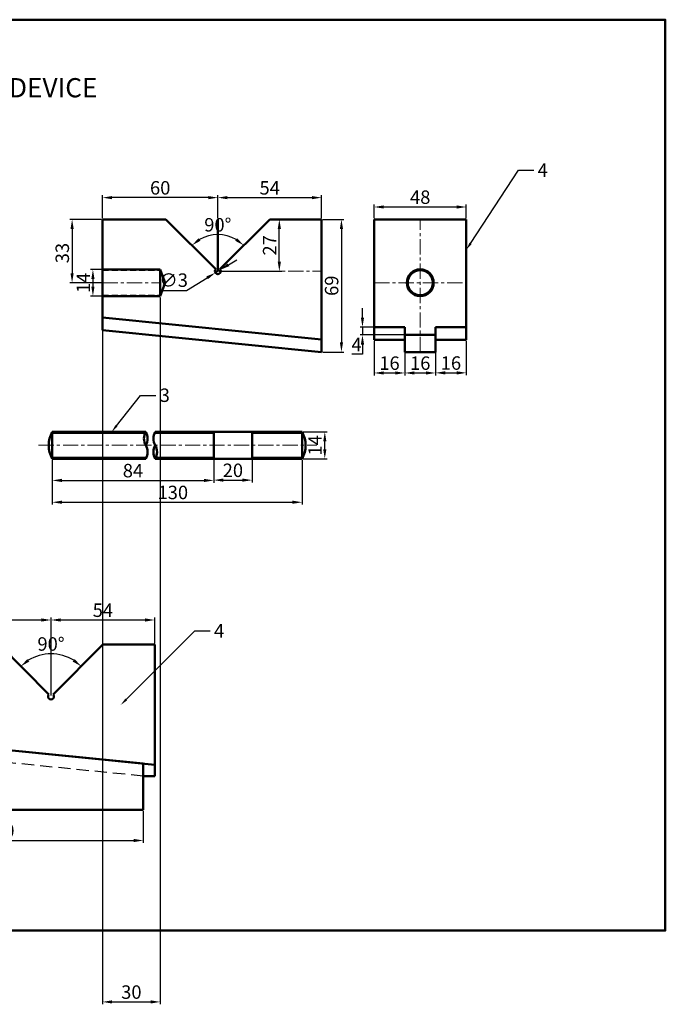
# Model space of a CAD drawing. Units: millimetres. Extents: x -238 to 500, y -191 to 322.
# Tile 3 of 3: x 164 to 500, y -191 to 322. Entities that reach past the tile are written whole.
import ezdxf
from ezdxf import colors
from ezdxf.entities.mleader import LeaderData, LeaderLine
from ezdxf.math import Vec2, Vec3

# ---------------------------------------------------------------- set-up
doc = ezdxf.new("R2010")
doc.units = ezdxf.units.MM
doc.header["$LTSCALE"] = 0.5
doc.linetypes.add('CENTER', pattern=[50.8, 31.75, -6.35, 6.35, -6.35])
doc.linetypes.add('DASHED', pattern=[19.05, 12.7, -6.35])
for name, color, linetype, lineweight in [('M-CNTR', 1, 'CENTER', 18), ('M-DIMS', 2, 'Continuous', 25), ('M-HIDN', 6, 'DASHED', 25), ('M-OUTL', 7, 'Continuous', 50), ('M-TEXT', 3, 'Continuous', 25), ('M-TTLB', 7, 'Continuous', 50)]:
    doc.layers.add(name, color=color, linetype=linetype, lineweight=lineweight)
doc.styles.get("Standard").update_dxf_attribs({"font": 'arial.ttf'})
doc.dimstyles.new('ISO-25', dxfattribs={"dimtxt": 7, "dimasz": 5, "dimexe": 1.25, "dimexo": 0.625, "dimtad": 1, "dimtoh": 1, "dimtxsty": 'Standard', "dimcen": 2.5, "dimadec": 0, "dimazin": 0, "dimtfac": 1, "dimtmove": 0, "dimatfit": 3, "dimfxl": 1, "dimarcsym": 0})

# ---------------------------------------------------------------- blocks, each defined once
blk = doc.blocks.new('*D1')
at = {"layer": 'Defpoints', "color": 0, "ltscale": 0.5, "transparency": 16777216}
for p in [(180.58, 93.15), (310.58, 93.15), (310.58, 70.53)]:
    blk.add_point(p, dxfattribs=at)
at = {"layer": 'M-DIMS', "color": 0, "lineweight": -2, "ltscale": 0.5, "transparency": 16777216}
for p, q in [((180.58, 92.53), (180.58, 69.28)), ((310.58, 92.53), (310.58, 69.28)), ((185.58, 70.53), (305.58, 70.53))]:
    blk.add_line(p, q, dxfattribs=at)
at = {"layer": 'M-DIMS', "color": 0, "ltscale": 0.5, "transparency": 16777216}
for points in [[(185.58, 71.37), (185.58, 69.7), (180.58, 70.53)], [(305.58, 71.37), (305.58, 69.7), (310.58, 70.53)]]:
    blk.add_solid(points, dxfattribs=at)
at = {"layer": 'M-DIMS', "color": 0, "ltscale": 0.5, "transparency": 16777216, "insert": (243.32, 74.73), "char_height": 7, "attachment_point": 5}
blk.add_mtext('130', dxfattribs=at)
blk = doc.blocks.new('*D2')
at = {"layer": 'Defpoints', "color": 0, "ltscale": 0.5, "transparency": 16777216}
for p in [(264.58, 93.15), (284.58, 93.15), (284.58, 82.04)]:
    blk.add_point(p, dxfattribs=at)
at = {"layer": 'M-DIMS', "color": 0, "lineweight": -2, "ltscale": 0.5, "transparency": 16777216}
for p, q in [((264.58, 92.53), (264.58, 80.79)), ((284.58, 92.53), (284.58, 80.79)), ((269.58, 82.04), (279.58, 82.04))]:
    blk.add_line(p, q, dxfattribs=at)
at = {"layer": 'M-DIMS', "color": 0, "ltscale": 0.5, "transparency": 16777216}
for points in [[(269.58, 82.87), (269.58, 81.21), (264.58, 82.04)], [(279.58, 82.87), (279.58, 81.21), (284.58, 82.04)]]:
    blk.add_solid(points, dxfattribs=at)
at = {"layer": 'M-DIMS', "color": 0, "ltscale": 0.5, "transparency": 16777216, "insert": (274.58, 86.24), "char_height": 7, "attachment_point": 5}
blk.add_mtext('20', dxfattribs=at)
blk = doc.blocks.new('*D3')
at = {"layer": 'Defpoints', "color": 0, "ltscale": 0.5, "transparency": 16777216}
for p in [(180.58, 93.15), (264.58, 93.15), (264.58, 81.89)]:
    blk.add_point(p, dxfattribs=at)
at = {"layer": 'M-DIMS', "color": 0, "lineweight": -2, "ltscale": 0.5, "transparency": 16777216}
for p, q in [((180.58, 92.53), (180.58, 80.64)), ((264.58, 92.53), (264.58, 80.64)), ((185.58, 81.89), (259.58, 81.89))]:
    blk.add_line(p, q, dxfattribs=at)
at = {"layer": 'M-DIMS', "color": 0, "ltscale": 0.5, "transparency": 16777216}
for points in [[(185.58, 82.72), (185.58, 81.05), (180.58, 81.89)], [(259.58, 82.72), (259.58, 81.05), (264.58, 81.89)]]:
    blk.add_solid(points, dxfattribs=at)
at = {"layer": 'M-DIMS', "color": 0, "ltscale": 0.5, "transparency": 16777216, "insert": (222.58, 86.08), "char_height": 7, "attachment_point": 5}
blk.add_mtext('84', dxfattribs=at)
blk = doc.blocks.new('*D4')
at = {"layer": 'Defpoints', "color": 0, "ltscale": 0.5, "transparency": 16777216}
for p in [(310.58, 107.15), (322.41, 107.15), (310.58, 93.15)]:
    blk.add_point(p, dxfattribs=at)
at = {"layer": 'M-DIMS', "color": 0, "lineweight": -2, "ltscale": 0.5, "transparency": 16777216}
for p, q in [((311.21, 107.15), (323.66, 107.15)), ((322.41, 98.15), (322.41, 102.15)), ((311.21, 93.15), (323.66, 93.15))]:
    blk.add_line(p, q, dxfattribs=at)
at = {"layer": 'M-DIMS', "color": 0, "ltscale": 0.5, "transparency": 16777216}
for points in [[(321.58, 102.15), (323.25, 102.15), (322.41, 107.15)], [(321.58, 98.15), (323.25, 98.15), (322.41, 93.15)]]:
    blk.add_solid(points, dxfattribs=at)
at = {"layer": 'M-DIMS', "color": 0, "ltscale": 0.5, "transparency": 16777216, "insert": (318.27, 100.15), "char_height": 7, "attachment_point": 5, "rotation": 90}
blk.add_mtext('14', dxfattribs=at)
blk = doc.blocks.new('*D32')
at = {"layer": 'Defpoints', "color": 0, "ltscale": 0.5, "transparency": 16777216}
for p in [(239.74, 217.71), (293.74, 217.71), (271.69, 209.15), (266.74, 190.71), (266.74, 190.71)]:
    blk.add_point(p, dxfattribs=at)
at = {"layer": 'M-DIMS', "color": 0, "lineweight": -2, "ltscale": 0.5, "transparency": 16777216}
blk.add_arc((266.74, 190.71), 19.09, 60.0485, 119.9515, dxfattribs=at)
at = {"layer": 'M-DIMS', "color": 0, "ltscale": 0.5, "transparency": 16777216}
for points in [[(257.72, 206.59), (256.71, 207.92), (253.24, 204.21)], [(276.78, 207.92), (275.77, 206.59), (280.24, 204.21)]]:
    blk.add_solid(points, dxfattribs=at)
at = {"layer": 'M-DIMS', "color": 0, "ltscale": 0.5, "transparency": 16777216, "insert": (266.74, 214), "char_height": 7, "attachment_point": 5}
blk.add_mtext('90°', dxfattribs=at)
blk = doc.blocks.new('*D33')
at = {"layer": 'Defpoints', "color": 0, "ltscale": 0.5, "transparency": 16777216}
for p in [(206.74, 229.03), (206.74, 217.71), (266.74, 217.71)]:
    blk.add_point(p, dxfattribs=at)
at = {"layer": 'M-DIMS', "color": 0, "lineweight": -2, "ltscale": 0.5, "transparency": 16777216}
for p, q in [((206.74, 218.34), (206.74, 230.28)), ((261.74, 229.03), (211.74, 229.03)), ((266.74, 218.34), (266.74, 230.28))]:
    blk.add_line(p, q, dxfattribs=at)
at = {"layer": 'M-DIMS', "color": 0, "ltscale": 0.5, "transparency": 16777216}
for points in [[(211.74, 229.87), (211.74, 228.2), (206.74, 229.03)], [(261.74, 229.87), (261.74, 228.2), (266.74, 229.03)]]:
    blk.add_solid(points, dxfattribs=at)
at = {"layer": 'M-DIMS', "color": 0, "ltscale": 0.5, "transparency": 16777216, "insert": (236.74, 233.23), "char_height": 7, "attachment_point": 5}
blk.add_mtext('60', dxfattribs=at)
blk = doc.blocks.new('*D34')
at = {"layer": 'Defpoints', "color": 0, "ltscale": 0.5, "transparency": 16777216}
for p in [(320.74, 229.03), (266.74, 217.71), (320.74, 217.71)]:
    blk.add_point(p, dxfattribs=at)
at = {"layer": 'M-DIMS', "color": 0, "lineweight": -2, "ltscale": 0.5, "transparency": 16777216}
for p, q in [((266.74, 218.34), (266.74, 230.28)), ((271.74, 229.03), (315.74, 229.03)), ((320.74, 218.34), (320.74, 230.28))]:
    blk.add_line(p, q, dxfattribs=at)
at = {"layer": 'M-DIMS', "color": 0, "ltscale": 0.5, "transparency": 16777216}
for points in [[(271.74, 229.87), (271.74, 228.2), (266.74, 229.03)], [(315.74, 229.87), (315.74, 228.2), (320.74, 229.03)]]:
    blk.add_solid(points, dxfattribs=at)
at = {"layer": 'M-DIMS', "color": 0, "ltscale": 0.5, "transparency": 16777216, "insert": (293.74, 233.22), "char_height": 7, "attachment_point": 5}
blk.add_mtext('54', dxfattribs=at)
blk = doc.blocks.new('*D35')
at = {"layer": 'Defpoints', "color": 0, "ltscale": 0.5, "transparency": 16777216}
for p in [(206.74, 217.71), (190.9, 184.71), (206.74, 184.71)]:
    blk.add_point(p, dxfattribs=at)
at = {"layer": 'M-DIMS', "color": 0, "lineweight": -2, "ltscale": 0.5, "transparency": 16777216}
for p, q in [((206.12, 217.71), (189.65, 217.71)), ((190.9, 212.71), (190.9, 189.71)), ((206.12, 184.71), (189.65, 184.71))]:
    blk.add_line(p, q, dxfattribs=at)
at = {"layer": 'M-DIMS', "color": 0, "ltscale": 0.5, "transparency": 16777216}
for points in [[(190.06, 212.71), (191.73, 212.71), (190.9, 217.71)], [(190.06, 189.71), (191.73, 189.71), (190.9, 184.71)]]:
    blk.add_solid(points, dxfattribs=at)
at = {"layer": 'M-DIMS', "color": 0, "ltscale": 0.5, "transparency": 16777216, "insert": (186.7, 200.19), "char_height": 7, "attachment_point": 5, "rotation": 90}
blk.add_mtext('33', dxfattribs=at)
blk = doc.blocks.new('*D36')
at = {"layer": 'Defpoints', "color": 0, "ltscale": 0.5, "transparency": 16777216}
for p in [(206.74, 191.71), (201.73, 177.71), (206.74, 177.71)]:
    blk.add_point(p, dxfattribs=at)
at = {"layer": 'M-DIMS', "color": 0, "lineweight": -2, "ltscale": 0.5, "transparency": 16777216}
for p, q in [((206.12, 191.71), (200.48, 191.71)), ((201.73, 186.71), (201.73, 182.71)), ((206.12, 177.71), (200.48, 177.71))]:
    blk.add_line(p, q, dxfattribs=at)
at = {"layer": 'M-DIMS', "color": 0, "ltscale": 0.5, "transparency": 16777216}
for points in [[(200.9, 186.71), (202.57, 186.71), (201.73, 191.71)], [(200.9, 182.71), (202.57, 182.71), (201.73, 177.71)]]:
    blk.add_solid(points, dxfattribs=at)
at = {"layer": 'M-DIMS', "color": 0, "ltscale": 0.5, "transparency": 16777216, "insert": (197.6, 184.71), "char_height": 7, "attachment_point": 5, "rotation": 90}
blk.add_mtext('14', dxfattribs=at)
blk = doc.blocks.new('*D37')
at = {"layer": 'Defpoints', "color": 0, "ltscale": 0.5, "transparency": 16777216}
for p in [(320.74, 217.71), (320.74, 148.71), (331.08, 148.71)]:
    blk.add_point(p, dxfattribs=at)
at = {"layer": 'M-DIMS', "color": 0, "lineweight": -2, "ltscale": 0.5, "transparency": 16777216}
for p, q in [((321.37, 217.71), (332.33, 217.71)), ((331.08, 212.71), (331.08, 153.71)), ((321.37, 148.71), (332.33, 148.71))]:
    blk.add_line(p, q, dxfattribs=at)
at = {"layer": 'M-DIMS', "color": 0, "ltscale": 0.5, "transparency": 16777216}
for points in [[(330.24, 212.71), (331.91, 212.71), (331.08, 217.71)], [(330.24, 153.71), (331.91, 153.71), (331.08, 148.71)]]:
    blk.add_solid(points, dxfattribs=at)
at = {"layer": 'M-DIMS', "color": 0, "ltscale": 0.5, "transparency": 16777216, "insert": (326.88, 183.21), "char_height": 7, "attachment_point": 5, "rotation": 90}
blk.add_mtext('69', dxfattribs=at)
blk = doc.blocks.new('*D38')
at = {"layer": 'Defpoints', "color": 0, "ltscale": 0.5, "transparency": 16777216}
for p in [(293.74, 217.71), (298.75, 217.71), (266.74, 190.71)]:
    blk.add_point(p, dxfattribs=at)
at = {"layer": 'M-DIMS', "color": 0, "lineweight": -2, "ltscale": 0.5, "transparency": 16777216}
for p, q in [((294.37, 217.71), (300, 217.71)), ((298.75, 195.71), (298.75, 212.71)), ((267.37, 190.71), (300, 190.71))]:
    blk.add_line(p, q, dxfattribs=at)
at = {"layer": 'M-DIMS', "color": 0, "ltscale": 0.5, "transparency": 16777216}
for points in [[(297.92, 212.71), (299.59, 212.71), (298.75, 217.71)], [(297.92, 195.71), (299.59, 195.71), (298.75, 190.71)]]:
    blk.add_solid(points, dxfattribs=at)
at = {"layer": 'M-DIMS', "color": 0, "ltscale": 0.5, "transparency": 16777216, "insert": (294.61, 204.21), "char_height": 7, "attachment_point": 5, "rotation": 90}
blk.add_mtext('27', dxfattribs=at)
blk = doc.blocks.new('*D39')
at = {"layer": 'Defpoints', "color": 0, "ltscale": 0.5, "transparency": 16777216}
for p in [(265.46, 189.93), (268.03, 191.49)]:
    blk.add_point(p, dxfattribs=at)
at = {"layer": 'M-DIMS', "color": 0, "lineweight": -2, "ltscale": 0.5, "transparency": 16777216}
for p, q in [((272.29, 194.1), (276.56, 196.7)), ((268.03, 191.49), (265.46, 189.93)), ((250.49, 180.8), (261.2, 187.33)), ((237.66, 180.8), (250.49, 180.8))]:
    blk.add_line(p, q, dxfattribs=at)
at = {"layer": 'M-DIMS', "color": 0, "ltscale": 0.5, "transparency": 16777216}
for points in [[(271.86, 194.81), (272.73, 193.39), (268.03, 191.49)], [(260.76, 188.04), (261.63, 186.62), (265.46, 189.93)]]:
    blk.add_solid(points, dxfattribs=at)
at = {"layer": 'M-DIMS', "color": 0, "ltscale": 0.5, "transparency": 16777216, "insert": (243.76, 185.2), "char_height": 7, "attachment_point": 5}
blk.add_mtext('∅3', dxfattribs=at)
blk = doc.blocks.new('*D40')
at = {"layer": 'Defpoints', "color": 0, "ltscale": 0.5, "transparency": 16777216}
for p in [(396.08, 224.17), (348.08, 217.71), (396.08, 217.71)]:
    blk.add_point(p, dxfattribs=at)
at = {"layer": 'M-DIMS', "color": 0, "lineweight": -2, "ltscale": 0.5, "transparency": 16777216}
for p, q in [((348.08, 218.34), (348.08, 225.42)), ((353.08, 224.17), (391.08, 224.17)), ((396.08, 218.34), (396.08, 225.42))]:
    blk.add_line(p, q, dxfattribs=at)
at = {"layer": 'M-DIMS', "color": 0, "ltscale": 0.5, "transparency": 16777216}
for points in [[(353.08, 225.01), (353.08, 223.34), (348.08, 224.17)], [(391.08, 225.01), (391.08, 223.34), (396.08, 224.17)]]:
    blk.add_solid(points, dxfattribs=at)
at = {"layer": 'M-DIMS', "color": 0, "ltscale": 0.5, "transparency": 16777216, "insert": (372.08, 228.37), "char_height": 7, "attachment_point": 5}
blk.add_mtext('48', dxfattribs=at)
blk = doc.blocks.new('*D41')
at = {"layer": 'Defpoints', "color": 0, "ltscale": 0.5, "transparency": 16777216}
for p in [(348.08, 161.58), (342.02, 157.58), (364.08, 157.58)]:
    blk.add_point(p, dxfattribs=at)
at = {"layer": 'M-DIMS', "color": 0, "lineweight": -2, "ltscale": 0.5, "transparency": 16777216}
for p, q in [((342.02, 166.58), (342.02, 171.58)), ((347.45, 161.58), (340.77, 161.58)), ((342.02, 161.58), (342.02, 157.58)), ((363.45, 157.58), (340.77, 157.58)), ((342.02, 152.58), (342.02, 147.58)), ((342.02, 147.58), (336.56, 147.58))]:
    blk.add_line(p, q, dxfattribs=at)
at = {"layer": 'M-DIMS', "color": 0, "ltscale": 0.5, "transparency": 16777216}
for points in [[(341.19, 166.58), (342.86, 166.58), (342.02, 161.58)], [(341.19, 152.58), (342.86, 152.58), (342.02, 157.58)]]:
    blk.add_solid(points, dxfattribs=at)
at = {"layer": 'M-DIMS', "color": 0, "ltscale": 0.5, "transparency": 16777216, "insert": (338.98, 151.71), "char_height": 7, "attachment_point": 5}
blk.add_mtext('4', dxfattribs=at)
blk = doc.blocks.new('*D42')
at = {"layer": 'Defpoints', "color": 0, "ltscale": 0.5, "transparency": 16777216}
for p in [(348.08, 155.08), (364.08, 155.08), (364.08, 137.8)]:
    blk.add_point(p, dxfattribs=at)
at = {"layer": 'M-DIMS', "color": 0, "lineweight": -2, "ltscale": 0.5, "transparency": 16777216}
for p, q in [((348.08, 154.46), (348.08, 136.55)), ((364.08, 154.46), (364.08, 136.55)), ((353.08, 137.8), (359.08, 137.8))]:
    blk.add_line(p, q, dxfattribs=at)
at = {"layer": 'M-DIMS', "color": 0, "ltscale": 0.5, "transparency": 16777216}
for points in [[(353.08, 138.64), (353.08, 136.97), (348.08, 137.8)], [(359.08, 138.64), (359.08, 136.97), (364.08, 137.8)]]:
    blk.add_solid(points, dxfattribs=at)
at = {"layer": 'M-DIMS', "color": 0, "ltscale": 0.5, "transparency": 16777216, "insert": (356.08, 142), "char_height": 7, "attachment_point": 5}
blk.add_mtext('16', dxfattribs=at)
blk = doc.blocks.new('*D43')
at = {"layer": 'Defpoints', "color": 0, "ltscale": 0.5, "transparency": 16777216}
for p in [(364.08, 148.71), (380.08, 148.71), (380.08, 137.8)]:
    blk.add_point(p, dxfattribs=at)
at = {"layer": 'M-DIMS', "color": 0, "lineweight": -2, "ltscale": 0.5, "transparency": 16777216}
for p, q in [((364.08, 148.09), (364.08, 136.55)), ((380.08, 148.09), (380.08, 136.55)), ((369.08, 137.8), (375.08, 137.8))]:
    blk.add_line(p, q, dxfattribs=at)
at = {"layer": 'M-DIMS', "color": 0, "ltscale": 0.5, "transparency": 16777216}
for points in [[(369.08, 138.64), (369.08, 136.97), (364.08, 137.8)], [(375.08, 138.64), (375.08, 136.97), (380.08, 137.8)]]:
    blk.add_solid(points, dxfattribs=at)
at = {"layer": 'M-DIMS', "color": 0, "ltscale": 0.5, "transparency": 16777216, "insert": (372.08, 142), "char_height": 7, "attachment_point": 5}
blk.add_mtext('16', dxfattribs=at)
blk = doc.blocks.new('*D44')
at = {"layer": 'Defpoints', "color": 0, "ltscale": 0.5, "transparency": 16777216}
for p in [(380.08, 155.15), (396.08, 155.15), (396.08, 137.86)]:
    blk.add_point(p, dxfattribs=at)
at = {"layer": 'M-DIMS', "color": 0, "lineweight": -2, "ltscale": 0.5, "transparency": 16777216}
for p, q in [((380.08, 154.52), (380.08, 136.61)), ((396.08, 154.52), (396.08, 136.61)), ((385.08, 137.86), (391.08, 137.86))]:
    blk.add_line(p, q, dxfattribs=at)
at = {"layer": 'M-DIMS', "color": 0, "ltscale": 0.5, "transparency": 16777216}
for points in [[(385.08, 138.69), (385.08, 137.02), (380.08, 137.86)], [(391.08, 138.69), (391.08, 137.02), (396.08, 137.86)]]:
    blk.add_solid(points, dxfattribs=at)
at = {"layer": 'M-DIMS', "color": 0, "ltscale": 0.5, "transparency": 16777216, "insert": (388.08, 142.06), "char_height": 7, "attachment_point": 5}
blk.add_mtext('16', dxfattribs=at)
blk = doc.blocks.new('*D48')
at = {"layer": 'Defpoints', "color": 0, "ltscale": 0.5, "transparency": 16777216}
for p in [(77.97, -89.46), (227.97, -89.46), (227.97, -105.49)]:
    blk.add_point(p, dxfattribs=at)
at = {"layer": 'M-DIMS', "color": 0, "lineweight": -2, "ltscale": 0.5, "transparency": 16777216}
for p, q in [((77.97, -90.09), (77.97, -106.74)), ((227.97, -90.09), (227.97, -106.74)), ((82.97, -105.49), (222.97, -105.49))]:
    blk.add_line(p, q, dxfattribs=at)
at = {"layer": 'M-DIMS', "color": 0, "ltscale": 0.5, "transparency": 16777216}
for points in [[(82.97, -104.66), (82.97, -106.32), (77.97, -105.49)], [(222.97, -104.66), (222.97, -106.32), (227.97, -105.49)]]:
    blk.add_solid(points, dxfattribs=at)
at = {"layer": 'M-DIMS', "color": 0, "ltscale": 0.5, "transparency": 16777216, "insert": (152.97, -101.29), "char_height": 7, "attachment_point": 5}
blk.add_mtext('150', dxfattribs=at)
blk = doc.blocks.new('*D49')
at = {"layer": 'Defpoints', "color": 0, "ltscale": 0.5, "transparency": 16777216}
for p in [(152.92, -3.57), (206.92, -3.57), (185.67, -9.09), (178.86, -29.51), (180.98, -29.51)]:
    blk.add_point(p, dxfattribs=at)
at = {"layer": 'M-DIMS', "color": 0, "lineweight": -2, "ltscale": 0.5, "transparency": 16777216}
blk.add_arc((179.92, -30.57), 22.24, 57.9107, 122.0893, dxfattribs=at)
at = {"layer": 'M-DIMS', "color": 0, "ltscale": 0.5, "transparency": 16777216}
for points in [[(168.62, -12.38), (167.58, -11.08), (164.19, -14.85)], [(192.25, -11.08), (191.21, -12.38), (195.64, -14.85)]]:
    blk.add_solid(points, dxfattribs=at)
at = {"layer": 'M-DIMS', "color": 0, "ltscale": 0.5, "transparency": 16777216, "insert": (179.92, -4.14), "char_height": 7, "attachment_point": 5}
blk.add_mtext('90°', dxfattribs=at)
blk = doc.blocks.new('*D50')
at = {"layer": 'Defpoints', "color": 0, "ltscale": 0.5, "transparency": 16777216}
for p in [(179.92, 9.26), (119.92, -3.57), (179.92, -30.57)]:
    blk.add_point(p, dxfattribs=at)
at = {"layer": 'M-DIMS', "color": 0, "lineweight": -2, "ltscale": 0.5, "transparency": 16777216}
for p, q in [((119.92, -2.95), (119.92, 10.51)), ((179.92, -29.95), (179.92, 10.51)), ((124.92, 9.26), (174.92, 9.26))]:
    blk.add_line(p, q, dxfattribs=at)
at = {"layer": 'M-DIMS', "color": 0, "ltscale": 0.5, "transparency": 16777216}
for points in [[(124.92, 10.09), (124.92, 8.42), (119.92, 9.26)], [(174.92, 10.09), (174.92, 8.42), (179.92, 9.26)]]:
    blk.add_solid(points, dxfattribs=at)
at = {"layer": 'M-DIMS', "color": 0, "ltscale": 0.5, "transparency": 16777216, "insert": (149.92, 13.46), "char_height": 7, "attachment_point": 5}
blk.add_mtext('60', dxfattribs=at)
blk = doc.blocks.new('*D51')
at = {"layer": 'Defpoints', "color": 0, "ltscale": 0.5, "transparency": 16777216}
for p in [(179.92, 9.26), (233.92, 9.26), (233.92, -3.57)]:
    blk.add_point(p, dxfattribs=at)
at = {"layer": 'M-DIMS', "color": 0, "lineweight": -2, "ltscale": 0.5, "transparency": 16777216}
for p, q in [((179.92, 9.88), (179.92, 10.51)), ((233.92, -2.95), (233.92, 10.51)), ((184.92, 9.26), (228.92, 9.26))]:
    blk.add_line(p, q, dxfattribs=at)
at = {"layer": 'M-DIMS', "color": 0, "ltscale": 0.5, "transparency": 16777216}
for points in [[(184.92, 10.09), (184.92, 8.42), (179.92, 9.26)], [(228.92, 10.09), (228.92, 8.42), (233.92, 9.26)]]:
    blk.add_solid(points, dxfattribs=at)
at = {"layer": 'M-DIMS', "color": 0, "ltscale": 0.5, "transparency": 16777216, "insert": (206.92, 13.44), "char_height": 7, "attachment_point": 5}
blk.add_mtext('54', dxfattribs=at)
blk = doc.blocks.new('*D53')
at = {"layer": 'Defpoints', "color": 0, "ltscale": 0.5, "transparency": 16777216}
for p in [(206.74, 177.71), (236.74, 177.71), (236.74, -189.48)]:
    blk.add_point(p, dxfattribs=at)
at = {"layer": 'M-DIMS', "color": 0, "lineweight": -2, "ltscale": 0.5, "transparency": 16777216}
for p, q in [((206.74, 177.09), (206.74, -190.73)), ((236.74, 177.09), (236.74, -190.73)), ((211.74, -189.48), (231.74, -189.48))]:
    blk.add_line(p, q, dxfattribs=at)
at = {"layer": 'M-DIMS', "color": 0, "ltscale": 0.5, "transparency": 16777216}
for points in [[(211.74, -188.65), (211.74, -190.31), (206.74, -189.48)], [(231.74, -188.65), (231.74, -190.31), (236.74, -189.48)]]:
    blk.add_solid(points, dxfattribs=at)
at = {"layer": 'M-DIMS', "color": 0, "ltscale": 0.5, "transparency": 16777216, "insert": (221.74, -185.28), "char_height": 7, "attachment_point": 5}
blk.add_mtext('30', dxfattribs=at)

msp = doc.modelspace()

# ---------------------------------------------------------------- linework, layer by layer
at = {"layer": 'M-CNTR', "ltscale": 0.5}
for p, q in [((372.077, 148.713), (372.077, 217.713)), ((265.245, 190.713), (320.745, 190.713)), ((206.745, 184.713), (236.745, 184.713)), ((348.077, 184.713), (396.077, 184.713)), ((173.464, 100.152), (318.355, 100.152))]:
    msp.add_line(p, q, dxfattribs=at)
at = {"layer": 'M-HIDN', "ltscale": 0.5}
for p, q in [((206.745, 191.213), (236.745, 191.213)), ((206.745, 178.213), (236.745, 178.213))]:
    msp.add_line(p, q, dxfattribs=at)
at = {"layer": 'M-HIDN'}
msp.add_line((227.969, -71.997), (119.916, -61.193), dxfattribs=at)
at = {"layer": 'M-OUTL', "ltscale": 0.5}
for p, q in [((206.745, 217.713), (239.745, 217.713)), ((206.745, 217.713), (206.745, 184.713)), ((265.684, 191.774), (239.745, 217.713)), ((266.745, 217.713), (266.745, 190.713)), ((267.805, 191.774), (293.745, 217.713)), ((293.745, 217.713), (320.745, 217.713)), ((320.745, 217.713), (320.745, 148.713)), ((348.077, 217.713), (396.077, 217.713)), ((348.077, 155.083), (348.077, 217.713)), ((396.077, 217.713), (396.077, 155.083)), ((206.745, 191.713), (236.745, 191.713)), ((236.745, 177.713), (236.745, 191.713)), ((236.745, 191.713), (239.293, 184.713)), ((206.745, 184.713), (206.745, 160.092)), ((236.745, 177.713), (239.293, 184.713)), ((206.745, 177.713), (236.745, 177.713)), ((320.745, 155.245), (206.745, 166.624)), ((320.745, 148.713), (206.745, 160.092)), ((348.077, 161.583), (364.077, 161.583)), ((364.077, 148.713), (364.077, 161.583)), ((380.077, 148.713), (380.077, 161.583)), ((380.077, 161.583), (396.077, 161.583)), ((348.077, 155.083), (364.077, 155.083)), ((364.077, 157.583), (380.077, 157.583)), ((380.077, 155.083), (396.077, 155.083)), ((380.077, 148.713), (364.077, 148.713)), ((180.581, 107.152), (229.207, 107.152)), ((180.581, 107.152), (180.581, 93.152)), ((180.581, 106.652), (228.944, 106.652)), ((233.92, 106.652), (264.581, 106.652)), ((234.182, 107.152), (310.581, 107.152)), ((264.581, 107.152), (264.581, 93.152)), ((284.581, 107.152), (284.581, 93.152)), ((284.581, 106.652), (310.581, 106.652)), ((310.581, 107.152), (310.581, 93.152)), ((180.581, 93.652), (229.469, 93.652)), ((180.581, 93.152), (229.207, 93.152)), ((234.182, 93.152), (310.581, 93.152)), ((234.445, 93.652), (264.581, 93.652)), ((284.581, 93.652), (310.581, 93.652)), ((178.855, -29.511), (152.916, -3.572)), ((180.976, -29.511), (206.916, -3.572)), ((206.916, -3.572), (233.916, -3.572)), ((233.916, -3.572), (233.916, -71.997)), ((233.916, -66.039), (119.916, -54.661)), ((227.969, -71.997), (233.916, -71.997))]:
    msp.add_line(p, q, dxfattribs=at)
at = {"layer": 'M-OUTL'}
for p, q in [((227.969, -65.465), (119.969, -54.666)), ((227.969, -89.465), (227.969, -65.465)), ((77.969, -89.465), (227.969, -89.465))]:
    msp.add_line(p, q, dxfattribs=at)
at = {"layer": 'M-OUTL', "ltscale": 0.5}
for radius in [7, 6.5]:
    msp.add_circle((372.077, 184.713), radius, dxfattribs=at)
for centre, radius, start, end in [((266.745, 190.713), 1.5, 135, 45), ((192.705, 100.152), 14, 150, 210), ((235.269, 103.652), 7, 150, 210), ((223.145, 103.652), 7, 330, 30), ((240.245, 103.652), 7, 150, 210), ((298.456, 100.152), 14, 330, 30), ((223.145, 96.652), 7, 330, 30), ((240.245, 96.652), 7, 150, 210), ((228.12, 96.652), 7, 330, 30), ((179.916, -30.572), 1.5, 135, 45)]:
    msp.add_arc(centre, radius, start, end, dxfattribs=at)
at = {"layer": 'M-TTLB', "ltscale": 0.5}
msp.add_lwpolyline([(-237.643, 321.636), (499.641, 321.636), (499.641, -152.379), (-237.643, -152.379)], close=True, dxfattribs=at)

# ---------------------------------------------------------------- texts
at = {"layer": 'M-TEXT', "ltscale": 0.5, "insert": (87.633, 291.237), "char_height": 10, "attachment_point": 1}
msp.add_mtext_dynamic_manual_height_columns('CLAMPING DEVICE', width=136.41378, gutter_width=12.5, heights=[0], dxfattribs=at)

# ---------------------------------------------------------------- dimensions: what is measured, and where the dimension line sits
at = {"layer": 'M-DIMS', "ltscale": 0.5}
for base, p1, p2, override, picture, middle in [((206.745, 229.033), (266.745, 217.713), (206.745, 217.713), {"dimclrd": 0, "dimclre": 0, "dimclrt": 0}, '*D33', (236.745, 233.232)), ((320.745, 229.033), (266.745, 217.713), (320.745, 217.713), {"dimclrd": 0, "dimclre": 0, "dimclrt": 0}, '*D34', (293.745, 233.217)), ((396.077, 224.172), (348.077, 217.713), (396.077, 217.713), {"dimclrd": 0, "dimclre": 0, "dimclrt": 0}, '*D40', (372.077, 228.371)), ((236.745, -189.479), (206.745, 177.713), (236.745, 177.713), {"dimdec": 0, "dimlfac": 1, "dimrnd": 0, "dimzin": 0, "dimdsep": 46, "dimlunit": 2}, '*D53', (221.745, -185.278)), ((364.077, 137.802), (348.077, 155.083), (364.077, 155.083), {"dimclrd": 0, "dimclre": 0, "dimclrt": 0}, '*D42', (356.077, 142.001)), ((396.077, 137.858), (380.077, 155.148), (396.077, 155.148), {"dimclrd": 0, "dimclre": 0, "dimclrt": 0}, '*D44', (388.077, 142.057)), ((284.581, 82.039), (264.581, 93.152), (284.581, 93.152), {"dimclrd": 0, "dimclre": 0, "dimclrt": 0}, '*D2', (274.581, 86.238)), ((179.916, 9.257), (119.916, -3.572), (179.916, -30.572), {"dimclrd": 0, "dimclre": 0, "dimclrt": 0}, '*D50', (149.916, 13.456)), ((233.916, 9.257), (179.916, 9.257), (233.916, -3.572), {"dimclrd": 0, "dimclre": 0, "dimclrt": 0}, '*D51', (206.916, 13.442)), ((227.969, -105.49), (77.969, -89.465), (227.969, -89.465), {"dimclrd": 0, "dimclre": 0, "dimclrt": 0}, '*D48', (152.969, -101.291))]:
    dim = msp.add_linear_dim(base=base, p1=p1, p2=p2, dimstyle='ISO-25', override=override, dxfattribs=at)
    dim.commit()
    dim.dimension.update_dxf_attribs({"geometry": picture, "text_midpoint": middle})
dim = msp.add_linear_dim(base=(190.898, 184.713), p1=(206.745, 217.713), p2=(206.745, 184.713), angle=90, dimstyle='ISO-25', override={"dimclrd": 0, "dimclre": 0, "dimclrt": 0}, dxfattribs=at)
dim.commit()
dim.dimension.update_dxf_attribs({"geometry": '*D35', "text_midpoint": (190.898, 200.194), "dimtype": 160})
for base, line1, line2, picture, middle in [((271.686, 209.154), ((266.745, 190.713), (293.745, 217.713)), ((266.745, 190.713), (239.745, 217.713)), '*D32', (266.745, 214.004)), ((185.671, -9.093), ((180.976, -29.511), (206.916, -3.572)), ((178.855, -29.511), (152.916, -3.572)), '*D49', (179.916, -4.136))]:
    dim = msp.add_angular_dim_2l(base=base, line1=line1, line2=line2, dimstyle='ISO-25', override={"dimclrd": 0, "dimclre": 0, "dimclrt": 0}, dxfattribs=at)
    dim.commit()
    dim.dimension.update_dxf_attribs({"geometry": picture, "text_midpoint": middle})
for base, p1, p2, picture, middle in [((298.753, 217.713), (266.745, 190.713), (293.745, 217.713), '*D38', (294.614, 204.213)), ((331.075, 148.713), (320.745, 217.713), (320.745, 148.713), '*D37', (326.876, 183.213)), ((201.735, 177.713), (206.745, 191.713), (206.745, 177.713), '*D36', (197.595, 184.713)), ((342.023, 157.583), (348.077, 161.583), (364.077, 157.583), '*D41', (338.977, 151.708)), ((322.413, 107.152), (310.581, 93.152), (310.581, 107.152), '*D4', (318.273, 100.152))]:
    dim = msp.add_linear_dim(base=base, p1=p1, p2=p2, angle=90, dimstyle='ISO-25', override={"dimclrd": 0, "dimclre": 0, "dimclrt": 0}, dxfattribs=at)
    dim.commit()
    dim.dimension.update_dxf_attribs({"geometry": picture, "text_midpoint": middle})
dim = msp.add_diameter_dim_2p(p1=(268.026, 191.494), p2=(265.464, 189.932), dimstyle='ISO-25', override={"dimclrd": 0, "dimclre": 0, "dimclrt": 0}, dxfattribs=at)
dim.commit()
dim.dimension.update_dxf_attribs({"geometry": '*D39', "text_midpoint": (243.761, 185.196)})
for base, p1, p2, picture, middle in [((380.077, 137.802), (364.077, 148.713), (380.077, 148.713), '*D43', (372.077, 137.802)), ((310.581, 70.532), (180.581, 93.152), (310.581, 93.152), '*D1', (243.323, 70.532)), ((264.581, 81.885), (180.581, 93.152), (264.581, 93.152), '*D3', (222.581, 81.885))]:
    dim = msp.add_linear_dim(base=base, p1=p1, p2=p2, dimstyle='ISO-25', override={"dimclrd": 0, "dimclre": 0, "dimclrt": 0}, dxfattribs=at)
    dim.commit()
    dim.dimension.update_dxf_attribs({"geometry": picture, "text_midpoint": middle, "dimtype": 160})

# ---------------------------------------------------------------- leaders
at = {"layer": 'M-TEXT', "ltscale": 0.5}
ml = msp.add_multileader_mtext('Standard', dxfattribs=at)
ml.set_content('4', color=256)
ml.set_leader_properties()
ml.build(insert=Vec2(0, 0))
ctx = ml.context
ctx.base_point, ctx.char_height, ctx.plane_origin = Vec3(431.153, 243.35), 7, Vec3(396.077, 201.893)
notes = []
notes.append((ctx, [(0, (1, 1, 0), (423.153, 243.35), (1, 0), 8, [(0, [(396.077, 201.893)], 0, [])])]))
ctx.mtext.insert, ctx.mtext.flow_direction = Vec3(433.153, 246.85), 5
ml = msp.add_multileader_mtext('Standard', dxfattribs=at)
ml.set_content('3', color=256)
ml.set_leader_properties()
ml.build(insert=Vec2(0, 0))
ctx = ml.context
ctx.base_point, ctx.char_height, ctx.plane_origin = Vec3(234.483, 126.154), 7, Vec3(211.51, 107.152)
notes.append((ctx, [(0, (1, 1, 0), (226.483, 126.154), (1, 0), 8, [(0, [(211.51, 107.152)], 0, [])])]))
ctx.mtext.insert, ctx.mtext.flow_direction = Vec3(236.483, 129.716), 5
ml = msp.add_multileader_mtext('Standard', dxfattribs=at)
ml.set_content('4', color=256)
ml.set_leader_properties()
ml.build(insert=Vec2(0, 0))
ctx = ml.context
ctx.base_point, ctx.char_height, ctx.plane_origin = Vec3(262.77, 3.611), 7, Vec3(216.221, -34.938)
notes.append((ctx, [(0, (1, 1, 0), (254.77, 3.611), (1, 0), 8, [(0, [(216.221, -34.938)], 0, [])])]))
ctx.mtext.insert, ctx.mtext.flow_direction = Vec3(264.77, 7.111), 5
for ctx, leaders in notes:
    for number, flags, end, landing, length, lines in leaders:
        leader = LeaderData()
        leader.index, (leader.has_last_leader_line, leader.has_dogleg_vector, leader.attachment_direction) = number, flags
        leader.last_leader_point, leader.dogleg_vector, leader.dogleg_length = Vec3(end), Vec3(landing), length
        for number, points, colour, breaks in lines:
            line = LeaderLine()
            line.index, line.vertices, line.color, line.breaks = number, Vec3.list(points), colors.encode_raw_color(colour), breaks
            leader.lines.append(line)
        ctx.leaders.append(leader)

doc.saveas('drawing.dxf')
